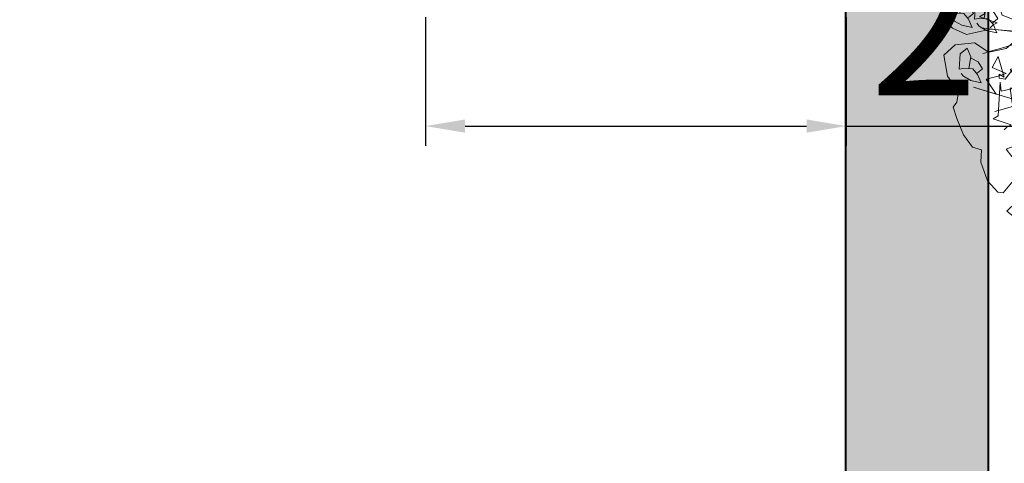
# Model space of a CAD drawing. Units: inches. Extents: x 2337 to 3570, y 1258 to 1938.
# Tile 8 of 30: x 2812 to 2874, y 1598 to 1626. Entities that reach past the tile are written whole.
import ezdxf

# ---------------------------------------------------------------- set-up
doc = ezdxf.new("R2010")
doc.units = ezdxf.units.IN
for name, color, linetype, lineweight in [('A-ANNO-DIMS', 2, 'Continuous', 18), ('A-WALL', 7, 'Continuous', 40), ('ARBOL', 74, 'Continuous', 13)]:
    doc.layers.add(name, color=color, linetype=linetype, lineweight=lineweight)
doc.layers.add('A-WALL-PATT', color=18, linetype='Continuous', lineweight=13, true_color=0x000000)
doc.layers.add('TALLO', color=36, linetype='Continuous')
doc.styles.get("Standard").update_dxf_attribs({"font": 'arial.ttf'})
doc.dimstyles.new('ISO-25', dxfattribs={"dimtxt": 9, "dimasz": 2.5, "dimexe": 1.25, "dimexo": 0.625, "dimtad": 1, "dimdec": 1, "dimlunit": 3, "dimtxsty": 'Standard', "dimcen": 2.5, "dimadec": 0, "dimazin": 0, "dimtfac": 1, "dimtdec": 1, "dimtmove": 0, "dimatfit": 3, "dimfxl": 1, "dimarcsym": 0})

# ---------------------------------------------------------------- blocks, each defined once
blk = doc.blocks.new('fresno')
at = {"layer": 'ARBOL'}
for p, q in [((2.96, 0.991), (3.575, 1.984)), ((-3.638, 1.194), (-4.164, 1.76)), ((-1.151, -0.932), (-1.99, -1.556)), ((-0.974, -3.757), (-1.31, -4.423))]:
    blk.add_line(p, q, dxfattribs=at)
blk.add_lwpolyline([(0.823, 4.745), (0.566, 4.764), (0.459, 4.687), (0.336, 4.518), (0.233, 4.322), (0.087, 4.298), (0.091, 4.464), (0.14, 4.621), (-0.09, 4.659), (-0.033, 4.863), (-0.264, 4.901), (-0.483, 4.866), (-0.686, 4.924), (-1.021, 4.801), (-1.288, 4.8), (-1.431, 4.563), (-1.234, 4.327), (-1.406, 4), (-1.205, 3.778), (-0.909, 3.705), (-0.931, 3.283), (-1.122, 2.983), (-1.491, 3.043), (-1.619, 3.562), (-1.9, 3.727), (-1.851, 3.982), (-2.197, 4.084), (-2.278, 4.31), (-2.543, 4.283), (-2.896, 4.152), (-3.091, 3.971), (-3.022, 3.817), (-3.244, 3.617), (-3.424, 3.528), (-3.697, 3.455), (-3.946, 3.236), (-3.922, 3.09), (-3.94, 2.548), (-3.617, 2.495), (-3.927, 2.19), (-4.062, 2.379), (-4.443, 2.512), (-4.546, 2.316), (-4.73, 2.062), (-4.767, 1.832), (-4.671, 1.698), (-4.486, 1.667), (-4.693, 1.559), (-4.854, 1.444), (-4.934, 1.102), (-5.037, 0.905), (-5.175, 0.644), (-5.166, 0.406), (-5.024, 0.264), (-4.781, 0.153), (-4.363, 0.249), (-4.014, 0.215), (-3.783, 0.177), (-3.46, 0.124), (-3.733, 0.051), (-4.132, -0.073), (-4.404, -0.146), (-4.639, 0.011), (-4.977, -0.028), (-5.172, -0.209), (-5.113, -0.574), (-4.921, -0.843), (-4.951, -1.027), (-5.012, -1.112), (-4.95, -1.311), (-4.83, -1.592), (-4.676, -1.807), (-4.518, -1.856), (-4.529, -2.068), (-4.417, -2.394), (-4.236, -2.59), (-4.143, -2.605), (-3.967, -2.397), (-3.703, -2.37), (-3.339, -2.027), (-3.032, -1.889), (-3.169, -2.15), (-3.115, -2.396), (-3.376, -2.542), (-3.552, -2.466), (-3.909, -2.762), (-4.077, -2.924), (-3.804, -3.135), (-3.592, -3.43), (-3.461, -3.499), (-3.253, -3.676), (-2.953, -3.867), (-2.792, -3.752), (-2.642, -3.848), (-2.572, -4.001), (-2.323, -4.066), (-2.18, -4.208), (-1.926, -4.392), (-1.58, -4.591), (-1.288, -4.545), (-1.027, -4.683), (-0.788, -4.675), (-0.531, -4.693), (-0.382, -4.505), (-0.29, -4.236), (-0.66, -3.891), (-0.588, -3.595), (-0.374, -3.441), (-0.267, -3.079), (-0.368, -2.541), (-0.208, -2.426), (-0.099, -2.633), (-0.087, -2.991), (0.071, -3.04), (0.129, -3.405), (-0.185, -3.59), (-0.119, -3.909), (0.055, -4.151), (0.136, -4.377), (0.456, -4.596), (0.828, -4.491), (1.227, -4.368), (1.461, -4.241), (1.583, -4.071), (1.748, -4.075), (1.86, -4.117), (2.101, -3.944), (2.308, -3.836), (2.925, -3.393), (3.101, -3.185), (2.74, -3.078), (2.812, -2.782), (2.769, -2.61), (3.015, -2.555), (3.012, -2.721), (3.254, -2.832), (3.546, -2.785), (3.752, -2.393), (3.882, -2.177), (3.92, -1.947), (4.069, -1.758), (4.214, -1.451), (4.144, -1.297), (4.021, -1.182), (4.182, -1.067), (4.304, -0.897), (4.464, -0.497), (4.429, -0.279), (4.406, -0.133), (3.964, -0.083), (3.074, -0.315), (2.582, -0.424), (2.217, -0.197), (2.136, 0.029), (2.462, 0.141), (2.628, -0.147), (3.012, -0.116), (3.249, 0.177), (3.602, 0.308), (3.701, 0.623), (4.089, 0.535), (4.404, 0.436), (4.464, 0.805), (4.272, 1.074), (4.267, 1.193), (4.336, 1.324), (4.243, 1.623), (4.092, 2.003), (3.769, 2.057), (3.485, 2.056), (3.642, 2.291), (3.88, 2.299), (3.71, 2.706), (3.563, 2.967), (3.201, 3.358), (3.001, 3.581), (2.766, 3.738), (2.635, 3.807), (2.332, 3.549), (2.268, 3.299), (2.052, 3.429), (2.136, 3.652), (1.798, 3.613), (1.437, 3.72), (1.755, 4.071), (1.513, 4.182), (1.451, 4.381), (1.519, 4.512), (1.204, 4.611), (1.012, 4.596)], close=True, dxfattribs=at)
for points in [[(-1.104, 4.45), (-1.063, 4.399), (-0.939, 4.325), (-0.757, 4.285), (-0.82, 4.431), (-0.903, 4.527), (-1.075, 4.533), (-1.143, 4.521), (-1.126, 4.792), (-1.002, 4.891), (-0.939, 4.738), (-0.975, 4.535)], [(-0.346, 4.735), (-0.501, 4.528), (-0.605, 4.545), (-0.605, 4.614), (-0.519, 4.563), (-0.622, 4.925), (-0.726, 4.735), (-0.484, 4.632), (-0.622, 4.58), (-0.829, 4.528), (-0.657, 4.27), (-1.053, 4.39), (-0.363, 4.183), (-0.381, 4.114), (-0.415, 4.373), (-0.26, 4.39), (-0.57, 4.321), (-0.588, 4.476), (-0.622, 3.89), (-0.708, 3.839), (-0.398, 3.735), (-0.467, 3.701), (-0.519, 3.649)], [(-0.935, 4.717), (-0.809, 4.65), (-0.736, 4.529), (-0.824, 4.459)], [(0.734, 4.203), (0.775, 4.152), (0.9, 4.078), (1.082, 4.038), (1.018, 4.185), (0.936, 4.281), (0.763, 4.287), (0.696, 4.274), (0.712, 4.546), (0.837, 4.645), (0.899, 4.491), (0.863, 4.289)], [(-0.521, 4.069), (-0.48, 4.018), (-0.356, 3.944), (-0.174, 3.904), (-0.237, 4.051), (-0.32, 4.146), (-0.492, 4.152), (-0.56, 4.14), (-0.543, 4.411), (-0.419, 4.511), (-0.356, 4.357), (-0.392, 4.154)], [(0.263, 4.114), (0.304, 4.063), (0.429, 3.989), (0.611, 3.948), (0.547, 4.095), (0.465, 4.191), (0.293, 4.197), (0.225, 4.185), (0.242, 4.456), (0.366, 4.555), (0.428, 4.402), (0.393, 4.199)], [(0.904, 4.471), (1.029, 4.404), (1.102, 4.282), (1.015, 4.212)], [(-1.623, 4.132), (-1.778, 3.925), (-1.882, 3.942), (-1.882, 4.011), (-1.795, 3.959), (-1.899, 4.321), (-2.002, 4.132), (-1.761, 4.028), (-1.899, 3.977), (-2.106, 3.925), (-1.933, 3.666), (-2.33, 3.787), (-1.64, 3.58), (-1.657, 3.511), (-1.692, 3.77), (-1.537, 3.787), (-1.847, 3.718), (-1.864, 3.873), (-1.899, 3.287), (-1.985, 3.235), (-1.675, 3.132), (-1.744, 3.097), (-1.795, 3.046)], [(-0.352, 4.337), (-0.226, 4.269), (-0.153, 4.148), (-0.241, 4.078)], [(0.433, 4.381), (0.558, 4.314), (0.631, 4.193), (0.544, 4.122)], [(-2.368, 4.073), (-2.523, 3.866), (-2.627, 3.883), (-2.627, 3.952), (-2.541, 3.9), (-2.644, 4.262), (-2.748, 4.073), (-2.506, 3.969), (-2.644, 3.918), (-2.851, 3.866), (-2.679, 3.607), (-3.075, 3.728), (-2.385, 3.521), (-2.403, 3.452), (-2.437, 3.711), (-2.282, 3.728), (-2.592, 3.659), (-2.61, 3.814), (-2.644, 3.228), (-2.73, 3.176), (-2.42, 3.073), (-2.489, 3.038), (-2.541, 2.987)], [(-2.629, 3.733), (-2.588, 3.682), (-2.463, 3.608), (-2.281, 3.568), (-2.345, 3.715), (-2.427, 3.81), (-2.6, 3.816), (-2.667, 3.804), (-2.651, 4.075), (-2.526, 4.175), (-2.464, 4.021), (-2.5, 3.818)], [(-1.149, 3.822), (-1.108, 3.771), (-0.983, 3.697), (-0.802, 3.657), (-0.865, 3.804), (-0.948, 3.9), (-1.12, 3.906), (-1.188, 3.893), (-1.171, 4.165), (-1.047, 4.264), (-0.984, 4.111), (-1.02, 3.908)], [(0.413, 4.08), (0.258, 3.873), (0.154, 3.89), (0.154, 3.959), (0.241, 3.908), (0.137, 4.27), (0.034, 4.08), (0.275, 3.977), (0.137, 3.925), (-0.07, 3.873), (0.103, 3.614), (-0.294, 3.735), (0.396, 3.528), (0.379, 3.459), (0.344, 3.718), (0.499, 3.735), (0.189, 3.666), (0.172, 3.821), (0.137, 3.235), (0.051, 3.183), (0.361, 3.08), (0.292, 3.046), (0.241, 2.994)], [(1.189, 3.942), (1.034, 3.735), (0.931, 3.752), (0.931, 3.821), (1.017, 3.77), (0.913, 4.132), (0.81, 3.942), (1.051, 3.839), (0.913, 3.787), (0.706, 3.735), (0.879, 3.477), (0.482, 3.597), (1.172, 3.39), (1.155, 3.321), (1.12, 3.58), (1.276, 3.597), (0.965, 3.528), (0.948, 3.683), (0.913, 3.097), (0.827, 3.046), (1.138, 2.942), (1.069, 2.908), (1.017, 2.856)], [(1.259, 4.08), (1.103, 3.873), (1, 3.89), (1, 3.959), (1.086, 3.908), (0.982, 4.27), (0.879, 4.08), (1.12, 3.977), (0.982, 3.925), (0.775, 3.873), (0.948, 3.614), (0.551, 3.735), (1.241, 3.528), (1.224, 3.459), (1.189, 3.718), (1.345, 3.735), (1.034, 3.666), (1.017, 3.821), (0.982, 3.235), (0.896, 3.183), (1.207, 3.08), (1.138, 3.046), (1.086, 2.994)], [(-2.459, 4), (-2.334, 3.933), (-2.261, 3.812), (-2.348, 3.742)], [(-0.287, 3.833), (-0.442, 3.626), (-0.546, 3.643), (-0.546, 3.712), (-0.46, 3.661), (-0.563, 4.023), (-0.667, 3.833), (-0.425, 3.73), (-0.563, 3.678), (-0.77, 3.626), (-0.598, 3.367), (-0.995, 3.488), (-0.304, 3.281), (-0.322, 3.212), (-0.356, 3.471), (-0.201, 3.488), (-0.511, 3.419), (-0.529, 3.574), (-0.563, 2.988), (-0.649, 2.936), (-0.339, 2.833), (-0.408, 2.799), (-0.46, 2.747)], [(-0.98, 4.09), (-0.854, 4.023), (-0.781, 3.901), (-0.869, 3.831)], [(1.25, 3.643), (1.291, 3.592), (1.416, 3.518), (1.597, 3.478), (1.534, 3.625), (1.451, 3.721), (1.279, 3.727), (1.211, 3.714), (1.228, 3.985), (1.352, 4.085), (1.415, 3.931), (1.379, 3.729)], [(-1.951, 3.597), (-2.106, 3.39), (-2.209, 3.408), (-2.209, 3.477), (-2.123, 3.425), (-2.227, 3.787), (-2.33, 3.597), (-2.089, 3.494), (-2.227, 3.442), (-2.434, 3.39), (-2.261, 3.132), (-2.658, 3.252), (-1.968, 3.046), (-1.985, 2.977), (-2.02, 3.235), (-1.864, 3.252), (-2.175, 3.183), (-2.192, 3.339), (-2.227, 2.752), (-2.313, 2.701), (-2.002, 2.597), (-2.071, 2.563), (-2.123, 2.511)], [(-2.068, 3.464), (-2.027, 3.413), (-1.903, 3.339), (-1.721, 3.299), (-1.784, 3.446), (-1.867, 3.542), (-2.039, 3.547), (-2.107, 3.535), (-2.09, 3.806), (-1.966, 3.906), (-1.903, 3.752), (-1.939, 3.55)], [(0.837, 2.414), (0.533, 3.352), (0.697, 3.906)], [(1.419, 3.911), (1.545, 3.844), (1.618, 3.722), (1.53, 3.652)], [(-2.898, 3.511), (-3.053, 3.304), (-3.157, 3.321), (-3.157, 3.39), (-3.071, 3.339), (-3.174, 3.701), (-3.278, 3.511), (-3.036, 3.408), (-3.174, 3.356), (-3.381, 3.304), (-3.209, 3.046), (-3.605, 3.166), (-2.915, 2.959), (-2.932, 2.89), (-2.967, 3.149), (-2.812, 3.166), (-3.122, 3.097), (-3.14, 3.253), (-3.174, 2.666), (-3.26, 2.615), (-2.95, 2.511), (-3.019, 2.477), (-3.071, 2.425)], [(-1.899, 3.732), (-1.773, 3.664), (-1.7, 3.543), (-1.788, 3.473)], [(-0.063, 3.671), (-0.069, 3.151), (-0.364, 2.965), (-0.319, 2.449)], [(1.259, 2.882), (1.254, 3.446), (1.381, 3.636)], [(-3.413, 3.083), (-3.373, 3.032), (-3.248, 2.958), (-3.066, 2.918), (-3.129, 3.065), (-3.212, 3.161), (-3.384, 3.167), (-3.452, 3.154), (-3.435, 3.425), (-3.311, 3.525), (-3.248, 3.371), (-3.284, 3.169)], [(-1.367, 2.367), (-1.081, 2.78), (-1.193, 3.514)], [(-0.923, 3.449), (-0.951, 3.425), (-0.93, 3.313)], [(-0.358, 2.895), (-0.615, 3.037), (-0.783, 3.596)], [(0.558, 3.402), (0.403, 3.195), (0.299, 3.212), (0.299, 3.281), (0.386, 3.23), (0.282, 3.592), (0.179, 3.402), (0.42, 3.299), (0.282, 3.247), (0.075, 3.195), (0.248, 2.936), (-0.149, 3.057), (0.541, 2.85), (0.524, 2.781), (0.489, 3.04), (0.644, 3.057), (0.334, 2.988), (0.317, 3.143), (0.282, 2.557), (0.196, 2.505), (0.506, 2.402), (0.437, 2.368), (0.386, 2.316)], [(1.564, 3.016), (1.605, 2.965), (1.729, 2.891), (1.911, 2.851), (1.848, 2.998), (1.765, 3.094), (1.593, 3.099), (1.525, 3.087), (1.542, 3.358), (1.666, 3.458), (1.729, 3.304), (1.693, 3.102)], [(2.191, 3.038), (2.232, 2.987), (2.357, 2.913), (2.539, 2.873), (2.475, 3.02), (2.393, 3.116), (2.221, 3.122), (2.153, 3.109), (2.17, 3.381), (2.294, 3.48), (2.356, 3.326), (2.321, 3.124)], [(2.573, 3.128), (2.613, 3.077), (2.738, 3.003), (2.92, 2.963), (2.857, 3.11), (2.774, 3.205), (2.602, 3.211), (2.534, 3.199), (2.551, 3.47), (2.675, 3.57), (2.738, 3.416), (2.702, 3.214)], [(-3.244, 3.351), (-3.118, 3.284), (-3.045, 3.162), (-3.133, 3.092)], [(-0.448, 1), (-0.961, 1.419), (-1.784, 3.341)], [(-0.41, 3.035), (-0.387, 2.974), (-0.291, 2.865), (-0.131, 2.771), (-0.146, 2.93), (-0.195, 3.047), (-0.357, 3.106), (-0.425, 3.115), (-0.325, 3.368), (-0.176, 3.424), (-0.164, 3.258), (-0.261, 3.077)], [(0.746, 2.242), (1.034, 2.786), (1.584, 3.019), (1.879, 3.374)], [(1.733, 3.284), (1.859, 3.216), (1.932, 3.095), (1.844, 3.025)], [(2.361, 3.306), (2.486, 3.239), (2.559, 3.117), (2.472, 3.047)], [(2.742, 3.396), (2.868, 3.328), (2.941, 3.207), (2.853, 3.137)], [(3.111, 2.904), (3.152, 2.853), (3.276, 2.779), (3.458, 2.739), (3.395, 2.886), (3.312, 2.981), (3.14, 2.987), (3.072, 2.975), (3.089, 3.246), (3.213, 3.346), (3.276, 3.192), (3.24, 2.99)], [(-2.225, 2.77), (-2.184, 2.718), (-2.06, 2.645), (-1.878, 2.604), (-1.941, 2.751), (-2.024, 2.847), (-2.196, 2.853), (-2.264, 2.84), (-2.247, 3.112), (-2.123, 3.211), (-2.06, 3.058), (-2.096, 2.855)], [(-1.575, 2.854), (-2.052, 2.969), (-2.2, 3.178)], [(-1.373, 2.77), (-1.332, 2.718), (-1.208, 2.645), (-1.026, 2.604), (-1.089, 2.751), (-1.172, 2.847), (-1.344, 2.853), (-1.412, 2.84), (-1.395, 3.112), (-1.271, 3.211), (-1.208, 3.058), (-1.244, 2.855)], [(-0.166, 3.238), (-0.068, 3.135), (-0.036, 2.997), (-0.141, 2.957)], [(2.326, 2.702), (2.367, 2.651), (2.492, 2.577), (2.673, 2.537), (2.61, 2.684), (2.527, 2.78), (2.355, 2.786), (2.287, 2.773), (2.304, 3.045), (2.428, 3.144), (2.491, 2.99), (2.455, 2.788)], [(3.28, 3.172), (3.406, 3.104), (3.479, 2.983), (3.391, 2.913)], [(-3.434, 2.752), (-3.59, 2.546), (-3.693, 2.563), (-3.693, 2.632), (-3.607, 2.58), (-3.71, 2.942), (-3.814, 2.752), (-3.572, 2.649), (-3.71, 2.597), (-3.917, 2.546), (-3.745, 2.287), (-4.142, 2.408), (-3.452, 2.201), (-3.469, 2.132), (-3.503, 2.39), (-3.348, 2.408), (-3.659, 2.339), (-3.676, 2.494), (-3.71, 1.908), (-3.797, 1.856), (-3.486, 1.753), (-3.555, 1.718), (-3.607, 1.666)], [(-1.112, 1.773), (-2.014, 2.265), (-2.654, 2.957)], [(-2.056, 3.037), (-1.93, 2.97), (-1.857, 2.849), (-1.945, 2.778)], [(-0.57, 2.77), (-0.726, 2.563), (-0.829, 2.58), (-0.829, 2.649), (-0.743, 2.597), (-0.846, 2.959), (-0.95, 2.77), (-0.708, 2.666), (-0.846, 2.615), (-1.053, 2.563), (-0.881, 2.304), (-1.278, 2.425), (-0.588, 2.218), (-0.605, 2.149), (-0.639, 2.408), (-0.484, 2.425), (-0.795, 2.356), (-0.812, 2.511), (-0.846, 1.925), (-0.933, 1.873), (-0.622, 1.77), (-0.691, 1.735), (-0.743, 1.684)], [(-1.204, 3.037), (-1.078, 2.97), (-1.005, 2.849), (-1.093, 2.778)], [(2.121, 2.804), (1.966, 2.597), (1.862, 2.615), (1.862, 2.683), (1.949, 2.632), (1.845, 2.994), (1.742, 2.804), (1.983, 2.701), (1.845, 2.649), (1.638, 2.597), (1.811, 2.339), (1.414, 2.459), (2.104, 2.252), (2.087, 2.184), (2.052, 2.442), (2.207, 2.459), (1.897, 2.39), (1.88, 2.546), (1.845, 1.959), (1.759, 1.908), (2.069, 1.804), (2, 1.77), (1.949, 1.718)], [(2.495, 2.97), (2.621, 2.903), (2.694, 2.781), (2.606, 2.711)], [(3.043, 2.478), (3.084, 2.427), (3.209, 2.353), (3.391, 2.313), (3.327, 2.46), (3.245, 2.556), (3.073, 2.562), (3.005, 2.549), (3.022, 2.82), (3.146, 2.92), (3.208, 2.766), (3.173, 2.564)], [(2.171, 1.674), (2.121, 2.172), (2.689, 2.898)], [(3.519, 2.666), (3.363, 2.459), (3.26, 2.477), (3.26, 2.546), (3.346, 2.494), (3.243, 2.856), (3.139, 2.666), (3.381, 2.563), (3.243, 2.511), (3.036, 2.459), (3.208, 2.201), (2.811, 2.321), (3.501, 2.115), (3.484, 2.046), (3.45, 2.304), (3.605, 2.321), (3.294, 2.252), (3.277, 2.408), (3.243, 1.821), (3.156, 1.77), (3.467, 1.666), (3.398, 1.632), (3.346, 1.58)], [(3.213, 2.746), (3.338, 2.679), (3.411, 2.557), (3.324, 2.487)], [(1.586, 2.528), (1.431, 2.321), (1.327, 2.339), (1.327, 2.408), (1.414, 2.356), (1.31, 2.718), (1.207, 2.528), (1.448, 2.425), (1.31, 2.373), (1.103, 2.321), (1.276, 2.063), (0.879, 2.184), (1.569, 1.977), (1.552, 1.908), (1.517, 2.166), (1.673, 2.184), (1.362, 2.115), (1.345, 2.27), (1.31, 1.684), (1.224, 1.632), (1.535, 1.528), (1.466, 1.494), (1.414, 1.442)], [(3.178, 2.165), (3.219, 2.113), (3.344, 2.04), (3.525, 1.999), (3.462, 2.146), (3.379, 2.242), (3.207, 2.248), (3.139, 2.236), (3.156, 2.507), (3.28, 2.606), (3.343, 2.453), (3.307, 2.25)], [(-4.422, 2.03), (-4.381, 1.979), (-4.257, 1.905), (-4.075, 1.865), (-4.138, 2.012), (-4.221, 2.108), (-4.393, 2.114), (-4.461, 2.101), (-4.444, 2.372), (-4.32, 2.472), (-4.257, 2.318), (-4.293, 2.116)], [(-3.468, 1.85), (-3.409, 2.222), (-3.628, 2.505)], [(-1.817, 2.351), (-1.972, 2.144), (-2.075, 2.162), (-2.075, 2.231), (-1.989, 2.179), (-2.093, 2.541), (-2.196, 2.351), (-1.955, 2.248), (-2.093, 2.196), (-2.3, 2.144), (-2.127, 1.886), (-2.524, 2.006), (-1.834, 1.8), (-1.851, 1.731), (-1.886, 1.989), (-1.73, 2.006), (-2.041, 1.937), (-2.058, 2.093), (-2.093, 1.506), (-2.179, 1.455), (-1.868, 1.351), (-1.937, 1.317), (-1.989, 1.265)], [(-1.786, 2.007), (-1.722, 1.99), (-1.578, 2.003), (-1.407, 2.078), (-1.545, 2.159), (-1.668, 2.188), (-1.811, 2.092), (-1.859, 2.042), (-2.004, 2.271), (-1.962, 2.425), (-1.821, 2.337), (-1.731, 2.152)], [(3.245, 1.963), (3.286, 1.912), (3.411, 1.838), (3.593, 1.798), (3.529, 1.945), (3.447, 2.041), (3.274, 2.046), (3.206, 2.034), (3.223, 2.305), (3.347, 2.405), (3.41, 2.251), (3.374, 2.049)], [(3.347, 2.432), (3.473, 2.365), (3.546, 2.244), (3.458, 2.173)], [(-3.986, 2.149), (-4.142, 1.942), (-4.245, 1.959), (-4.245, 2.028), (-4.159, 1.977), (-4.262, 2.339), (-4.366, 2.149), (-4.124, 2.046), (-4.262, 1.994), (-4.47, 1.942), (-4.297, 1.684), (-4.694, 1.804), (-4.004, 1.597), (-4.021, 1.528), (-4.055, 1.787), (-3.9, 1.804), (-4.211, 1.735), (-4.228, 1.89), (-4.262, 1.304), (-4.349, 1.253), (-4.038, 1.149), (-4.107, 1.115), (-4.159, 1.063)], [(-4.253, 2.298), (-4.127, 2.231), (-4.054, 2.109), (-4.142, 2.039)], [(-3.533, 2.149), (-3.43, 2.247), (-3.292, 2.279), (-3.252, 2.174)], [(-1.806, 2.323), (-1.665, 2.343), (-1.534, 2.287), (-1.564, 2.179)], [(-0.566, 1.873), (-0.525, 1.822), (-0.4, 1.748), (-0.219, 1.708), (-0.282, 1.855), (-0.365, 1.951), (-0.537, 1.957), (-0.605, 1.944), (-0.588, 2.216), (-0.464, 2.315), (-0.401, 2.162), (-0.437, 1.959)], [(3.415, 2.231), (3.54, 2.163), (3.613, 2.042), (3.525, 1.972)], [(-2.916, 0.958), (-3.096, 1.528), (-3.871, 2.197)], [(-3.331, 1.905), (-3.269, 1.928), (-3.161, 2.024), (-3.066, 2.184), (-3.226, 2.169), (-3.342, 2.121), (-3.401, 1.958), (-3.41, 1.89), (-3.663, 1.99), (-3.719, 2.139), (-3.554, 2.151), (-3.372, 2.054)], [(-1.164, 1.612), (-1.109, 1.576), (-0.967, 1.544), (-0.782, 1.562), (-0.888, 1.682), (-0.996, 1.748), (-1.162, 1.7), (-1.222, 1.667), (-1.29, 1.93), (-1.203, 2.063), (-1.096, 1.937), (-1.067, 1.733)], [(-0.397, 2.141), (-0.271, 2.074), (-0.198, 1.952), (-0.286, 1.882)], [(0.72, 1.798), (0.723, 1.733), (0.781, 1.6), (0.904, 1.46), (0.939, 1.616), (0.929, 1.742), (0.793, 1.848), (0.73, 1.878), (0.904, 2.088), (1.062, 2.095), (1.023, 1.934), (0.875, 1.791)], [(-2.965, 1.493), (-2.924, 1.441), (-2.799, 1.368), (-2.618, 1.327), (-2.681, 1.474), (-2.764, 1.57), (-2.936, 1.576), (-3.004, 1.564), (-2.987, 1.835), (-2.863, 1.934), (-2.8, 1.781), (-2.836, 1.578)], [(-1.085, 1.919), (-0.945, 1.893), (-0.838, 1.801), (-0.9, 1.707)], [(1.014, 1.915), (1.077, 1.787), (1.064, 1.646), (0.952, 1.64)], [(3.649, 1.515), (3.69, 1.464), (3.814, 1.39), (3.996, 1.35), (3.933, 1.497), (3.85, 1.592), (3.678, 1.598), (3.61, 1.586), (3.627, 1.857), (3.751, 1.957), (3.814, 1.803), (3.778, 1.601)], [(3.716, 1.537), (3.757, 1.486), (3.882, 1.412), (4.063, 1.372), (4, 1.519), (3.917, 1.615), (3.745, 1.621), (3.677, 1.608), (3.694, 1.88), (3.818, 1.979), (3.881, 1.825), (3.845, 1.623)], [(-2.796, 1.76), (-2.67, 1.693), (-2.597, 1.572), (-2.685, 1.501)], [(2.587, 1.684), (2.432, 1.477), (2.328, 1.494), (2.328, 1.563), (2.414, 1.511), (2.311, 1.873), (2.207, 1.684), (2.449, 1.58), (2.311, 1.528), (2.104, 1.477), (2.276, 1.218), (1.88, 1.339), (2.57, 1.132), (2.552, 1.063), (2.518, 1.321), (2.673, 1.339), (2.363, 1.27), (2.345, 1.425), (2.311, 0.839), (2.225, 0.787), (2.535, 0.684), (2.466, 0.649), (2.414, 0.597)], [(3.818, 1.783), (3.944, 1.715), (4.017, 1.594), (3.929, 1.524)], [(3.885, 1.805), (4.011, 1.738), (4.084, 1.616), (3.996, 1.546)], [(-4.193, 1.356), (-4.349, 1.149), (-4.452, 1.166), (-4.452, 1.235), (-4.366, 1.184), (-4.469, 1.546), (-4.573, 1.356), (-4.331, 1.253), (-4.469, 1.201), (-4.677, 1.149), (-4.504, 0.89), (-4.901, 1.011), (-4.211, 0.804), (-4.228, 0.735), (-4.262, 0.994), (-4.107, 1.011), (-4.418, 0.942), (-4.435, 1.097), (-4.469, 0.511), (-4.556, 0.459), (-4.245, 0.356), (-4.314, 0.322), (-4.366, 0.27)], [(-4.759, 1.269), (-4.718, 1.217), (-4.593, 1.144), (-4.411, 1.103), (-4.475, 1.25), (-4.557, 1.346), (-4.729, 1.352), (-4.797, 1.339), (-4.78, 1.611), (-4.656, 1.71), (-4.594, 1.557), (-4.629, 1.354)], [(-1.575, 1.269), (-1.534, 1.217), (-1.409, 1.144), (-1.228, 1.103), (-1.291, 1.25), (-1.373, 1.346), (-1.546, 1.352), (-1.614, 1.339), (-1.597, 1.611), (-1.473, 1.71), (-1.41, 1.557), (-1.446, 1.354)], [(1.283, 1.469), (1.266, 1.405), (1.279, 1.261), (1.354, 1.09), (1.435, 1.228), (1.464, 1.351), (1.368, 1.494), (1.318, 1.542), (1.547, 1.687), (1.7, 1.645), (1.613, 1.504), (1.428, 1.414)], [(3.761, 1.112), (3.802, 1.061), (3.926, 0.987), (4.108, 0.947), (4.045, 1.093), (3.962, 1.189), (3.79, 1.195), (3.722, 1.183), (3.739, 1.454), (3.863, 1.553), (3.926, 1.4), (3.89, 1.197)], [(-4.589, 1.536), (-4.464, 1.469), (-4.391, 1.348), (-4.478, 1.277)], [(-1.406, 1.536), (-1.28, 1.469), (-1.207, 1.348), (-1.295, 1.277)], [(0.308, 0.933), (0.349, 0.881), (0.474, 0.807), (0.656, 0.767), (0.592, 0.914), (0.51, 1.01), (0.337, 1.016), (0.27, 1.003), (0.286, 1.275), (0.411, 1.374), (0.473, 1.221), (0.437, 1.018)], [(1.599, 1.489), (1.618, 1.348), (1.563, 1.217), (1.455, 1.247)], [(2.479, 1.34), (2.443, 1.285), (2.411, 1.143), (2.429, 0.958), (2.549, 1.064), (2.615, 1.172), (2.567, 1.338), (2.534, 1.398), (2.797, 1.466), (2.93, 1.379), (2.804, 1.272), (2.6, 1.243)], [(3.139, 1.235), (2.984, 1.028), (2.88, 1.046), (2.88, 1.115), (2.967, 1.063), (2.863, 1.425), (2.759, 1.235), (3.001, 1.132), (2.863, 1.08), (2.656, 1.028), (2.828, 0.77), (2.432, 0.891), (3.122, 0.684), (3.105, 0.615), (3.07, 0.873), (3.225, 0.891), (2.915, 0.822), (2.897, 0.977), (2.863, 0.391), (2.777, 0.339), (3.087, 0.235), (3.018, 0.201), (2.967, 0.149)], [(3.93, 1.379), (4.056, 1.312), (4.129, 1.191), (4.041, 1.121)], [(-3.192, 1.017), (-3.578, 1.215), (-3.949, 1.081), (-4.398, 1.339)], [(-3.481, 0.843), (-3.44, 0.792), (-3.315, 0.718), (-3.133, 0.678), (-3.197, 0.825), (-3.279, 0.92), (-3.451, 0.926), (-3.519, 0.914), (-3.502, 1.185), (-3.378, 1.285), (-3.316, 1.131), (-3.351, 0.928)], [(-2.703, 1.201), (-2.575, 1.263), (-2.433, 1.251), (-2.428, 1.139)], [(2.786, 1.261), (2.76, 1.121), (2.668, 1.014), (2.574, 1.076)], [(4.01, 1.36), (3.422, 0.918)], [(4.26, 1.115), (4.105, 0.908), (4.002, 0.925), (4.002, 0.994), (4.088, 0.942), (3.984, 1.304), (3.881, 1.115), (4.122, 1.011), (3.984, 0.959), (3.777, 0.908), (3.95, 0.649), (3.553, 0.77), (4.243, 0.563), (4.226, 0.494), (4.191, 0.753), (4.347, 0.77), (4.036, 0.701), (4.019, 0.856), (3.984, 0.27), (3.898, 0.218), (4.209, 0.115), (4.14, 0.08), (4.088, 0.029)], [(-3.354, 1.176), (-4.529, 0.864)], [(-3.311, 1.111), (-3.186, 1.043), (-3.113, 0.922), (-3.2, 0.852)], [(0.478, 1.2), (0.603, 1.133), (0.676, 1.011), (0.589, 0.941)], [(2.808, 1.015), (3.422, 0.918), (3.422, 0.918), (3.748, 0.794), (4.154, 1.111)], [(-5.028, 0.44), (-4.987, 0.388), (-4.862, 0.315), (-4.68, 0.274), (-4.744, 0.421), (-4.826, 0.517), (-4.998, 0.523), (-5.066, 0.511), (-5.049, 0.782), (-4.925, 0.881), (-4.863, 0.728), (-4.898, 0.525)], [(-1.981, 0.615), (-1.915, 0.618), (-1.782, 0.676), (-1.643, 0.799), (-1.799, 0.834), (-1.925, 0.824), (-2.031, 0.688), (-2.061, 0.626), (-2.27, 0.799), (-2.278, 0.958), (-2.117, 0.918), (-1.974, 0.77)], [(-0.397, 0.517), (-0.346, 0.557), (-0.272, 0.682), (-0.232, 0.864), (-0.379, 0.801), (-0.474, 0.718), (-0.48, 0.546), (-0.468, 0.478), (-0.739, 0.495), (-0.838, 0.619), (-0.685, 0.682), (-0.482, 0.646)], [(4.075, 0.529), (4.116, 0.478), (4.24, 0.404), (4.422, 0.364), (4.359, 0.511), (4.276, 0.607), (4.104, 0.613), (4.036, 0.6), (4.053, 0.871), (4.177, 0.971), (4.24, 0.817), (4.204, 0.615)], [(-4.858, 0.707), (-4.733, 0.64), (-4.66, 0.519), (-4.747, 0.448)], [(-4.602, 0.35), (-4.561, 0.299), (-4.436, 0.225), (-4.254, 0.185), (-4.318, 0.332), (-4.4, 0.428), (-4.572, 0.433), (-4.64, 0.421), (-4.623, 0.692), (-4.499, 0.792), (-4.437, 0.638), (-4.472, 0.436)], [(-2.698, 0.509), (-2.854, 0.302), (-2.957, 0.319), (-2.957, 0.388), (-2.871, 0.336), (-2.974, 0.698), (-3.078, 0.509), (-2.836, 0.405), (-2.974, 0.353), (-3.182, 0.302), (-3.009, 0.043), (-3.406, 0.164), (-2.716, -0.043), (-2.733, -0.112), (-2.767, 0.147), (-2.612, 0.164), (-2.923, 0.095), (-2.94, 0.25), (-2.974, -0.336), (-3.061, -0.388), (-2.75, -0.491), (-2.819, -0.526), (-2.871, -0.577)], [(2.639, 0.58), (2.483, 0.373), (2.38, 0.391), (2.38, 0.46), (2.466, 0.408), (2.363, 0.77), (2.259, 0.58), (2.501, 0.477), (2.363, 0.425), (2.156, 0.373), (2.328, 0.115), (1.931, 0.235), (2.621, 0.029), (2.604, -0.04), (2.57, 0.218), (2.725, 0.235), (2.414, 0.166), (2.397, 0.322), (2.363, -0.265), (2.276, -0.316), (2.587, -0.42), (2.518, -0.454), (2.466, -0.506)], [(2.708, 0.563), (2.552, 0.356), (2.449, 0.373), (2.449, 0.442), (2.535, 0.391), (2.432, 0.753), (2.328, 0.563), (2.57, 0.46), (2.432, 0.408), (2.225, 0.356), (2.397, 0.097), (2, 0.218), (2.69, 0.011), (2.673, -0.058), (2.639, 0.201), (2.794, 0.218), (2.483, 0.149), (2.466, 0.304), (2.432, -0.282), (2.345, -0.334), (2.656, -0.437), (2.587, -0.471), (2.535, -0.523)], [(4.244, 0.797), (4.37, 0.73), (4.443, 0.608), (4.355, 0.538)], [(-4.432, 0.618), (-4.307, 0.55), (-4.234, 0.429), (-4.321, 0.359)], [(-3.824, 0.404), (-3.763, 0.427), (-3.654, 0.523), (-3.559, 0.683), (-3.719, 0.668), (-3.835, 0.62), (-3.894, 0.457), (-3.903, 0.389), (-4.156, 0.489), (-4.212, 0.638), (-4.047, 0.65), (-3.865, 0.553)], [(-2.322, 0.222), (-2.219, 0.321), (-2.081, 0.353), (-2.042, 0.248)], [(1.978, 0.384), (1.927, 0.343), (1.853, 0.218), (1.813, 0.036), (1.96, 0.1), (2.056, 0.182), (2.061, 0.355), (2.049, 0.422), (2.32, 0.406), (2.42, 0.281), (2.266, 0.219), (2.064, 0.254)], [(3.829, 0.184), (3.674, -0.023), (3.57, -0.006), (3.57, 0.063), (3.657, 0.011), (3.553, 0.373), (3.45, 0.184), (3.691, 0.08), (3.553, 0.029), (3.346, -0.023), (3.519, -0.282), (3.122, -0.161), (3.812, -0.368), (3.795, -0.437), (3.76, -0.178), (3.915, -0.161), (3.605, -0.23), (3.588, -0.075), (3.553, -0.661), (3.467, -0.713), (3.777, -0.816), (3.708, -0.851), (3.657, -0.902)], [(-3.394, 0.18), (-3.77, 0.182), (-4.532, 0.27)], [(-3.77, 0.182), (-4.09, -0.088), (-4.494, -0.18)], [(-0.596, -0.564), (0.03, -0.026), (0.339, 0.235)], [(2.246, 0.214), (2.178, 0.089), (2.057, 0.016), (1.987, 0.103)], [(-1.642, -0.412), (-1.601, -0.463), (-1.477, -0.537), (-1.295, -0.577), (-1.358, -0.43), (-1.441, -0.334), (-1.613, -0.328), (-1.681, -0.341), (-1.664, -0.069), (-1.54, 0.03), (-1.477, -0.124), (-1.513, -0.326)], [(0.03, -0.026), (-0.491, 0.154), (-0.871, -0.08)], [(0.38, 0.131), (0.248, -0.21), (-0.33, -0.951)], [(-4.871, -0.524), (-4.83, -0.575), (-4.705, -0.649), (-4.523, -0.689), (-4.587, -0.542), (-4.669, -0.446), (-4.841, -0.44), (-4.909, -0.453), (-4.893, -0.181), (-4.768, -0.082), (-4.706, -0.236), (-4.741, -0.438)], [(-1.473, -0.144), (-1.347, -0.211), (-1.274, -0.333), (-1.362, -0.403)], [(3.139, -0.282), (2.984, -0.489), (2.88, -0.471), (2.88, -0.402), (2.967, -0.454), (2.863, -0.092), (2.759, -0.282), (3.001, -0.385), (2.863, -0.437), (2.656, -0.489), (2.828, -0.747), (2.432, -0.627), (3.122, -0.834), (3.105, -0.902), (3.07, -0.644), (3.225, -0.627), (2.915, -0.696), (2.897, -0.54), (2.863, -1.127), (2.777, -1.178), (3.087, -1.282), (3.018, -1.316), (2.967, -1.368)], [(-4.701, -0.256), (-4.576, -0.323), (-4.503, -0.445), (-4.59, -0.515)], [(-3.952, -0.42), (-4.107, -0.627), (-4.211, -0.609), (-4.211, -0.54), (-4.124, -0.592), (-4.228, -0.23), (-4.331, -0.42), (-4.09, -0.523), (-4.228, -0.575), (-4.435, -0.627), (-4.262, -0.885), (-4.659, -0.765), (-3.969, -0.971), (-3.986, -1.04), (-4.021, -0.782), (-3.866, -0.765), (-4.176, -0.834), (-4.193, -0.678), (-4.228, -1.265), (-4.314, -1.316), (-4.004, -1.42), (-4.073, -1.454), (-4.124, -1.506)], [(-3.58, -0.559), (-3.529, -0.518), (-3.455, -0.393), (-3.415, -0.211), (-3.562, -0.275), (-3.658, -0.357), (-3.664, -0.53), (-3.651, -0.597), (-3.923, -0.581), (-4.022, -0.456), (-3.868, -0.394), (-3.666, -0.43)], [(-3.848, -0.389), (-3.781, -0.264), (-3.659, -0.191), (-3.589, -0.278)], [(1.822, -0.495), (2.859, -1.165)], [(1.846, -0.51), (2.605, -0.469), (3.129, -0.637)], [(-3.141, -0.713), (-3.296, -0.92), (-3.4, -0.902), (-3.4, -0.834), (-3.314, -0.885), (-3.417, -0.523), (-3.521, -0.713), (-3.279, -0.816), (-3.417, -0.868), (-3.624, -0.92), (-3.452, -1.178), (-3.848, -1.058), (-3.158, -1.265), (-3.175, -1.333), (-3.21, -1.075), (-3.055, -1.058), (-3.365, -1.127), (-3.383, -0.971), (-3.417, -1.558), (-3.503, -1.609), (-3.193, -1.713), (-3.262, -1.747), (-3.314, -1.799)], [(1.304, -0.681), (1.241, -0.664), (1.097, -0.678), (0.926, -0.752), (1.064, -0.833), (1.187, -0.862), (1.33, -0.766), (1.377, -0.716), (1.523, -0.945), (1.481, -1.099), (1.34, -1.011), (1.25, -0.826)], [(-3.195, -0.824), (-3.267, -0.898), (-4.285, -1.185)], [(-1.047, -0.767), (-1.151, -0.913), (-1.144, -1.307), (-1.61, -1.871)], [(-1.794, -1.268), (-1.758, -1.214), (-1.726, -1.072), (-1.744, -0.887), (-1.865, -0.993), (-1.93, -1.101), (-1.883, -1.266), (-1.85, -1.327), (-2.113, -1.395), (-2.246, -1.307), (-2.119, -1.2), (-1.916, -1.172)], [(-2.101, -1.19), (-2.076, -1.05), (-1.983, -0.943), (-1.889, -1.004)], [(-0.346, -1.024), (-1.05, -2.251)], [(1.903, -0.903), (1.837, -0.905), (1.704, -0.963), (1.565, -1.086), (1.721, -1.122), (1.847, -1.111), (1.953, -0.975), (1.983, -0.913), (2.192, -1.086), (2.2, -1.245), (2.039, -1.205), (1.896, -1.057)], [(0.748, -1.185), (1.452, -1.855), (2.021, -2.292)], [(2.02, -1.197), (1.891, -1.259), (1.75, -1.247), (1.745, -1.134)], [(3.253, -1.094), (3.192, -1.117), (3.083, -1.213), (2.988, -1.374), (3.148, -1.359), (3.264, -1.31), (3.323, -1.148), (3.332, -1.079), (3.585, -1.179), (3.641, -1.328), (3.476, -1.34), (3.294, -1.244)], [(3.105, -1.471), (2.949, -1.678), (2.846, -1.661), (2.846, -1.592), (2.932, -1.644), (2.829, -1.282), (2.725, -1.471), (2.967, -1.575), (2.829, -1.627), (2.621, -1.678), (2.794, -1.937), (2.397, -1.816), (3.087, -2.023), (3.07, -2.092), (3.036, -1.833), (3.191, -1.816), (2.88, -1.885), (2.863, -1.73), (2.829, -2.316), (2.742, -2.368), (3.053, -2.471), (2.984, -2.506), (2.932, -2.558)], [(3.455, -1.338), (3.352, -1.437), (3.214, -1.469), (3.175, -1.364)], [(-1.361, -1.756), (-1.343, -1.693), (-1.357, -1.548), (-1.431, -1.377), (-1.513, -1.515), (-1.542, -1.638), (-1.445, -1.781), (-1.395, -1.829), (-1.625, -1.974), (-1.778, -1.932), (-1.691, -1.791), (-1.506, -1.701)], [(-1.677, -1.776), (-1.696, -1.635), (-1.641, -1.504), (-1.533, -1.534)], [(-3.648, -1.948), (-3.596, -1.907), (-3.523, -1.782), (-3.482, -1.6), (-3.629, -1.664), (-3.725, -1.746), (-3.731, -1.919), (-3.719, -1.986), (-3.99, -1.97), (-4.089, -1.845), (-3.936, -1.783), (-3.733, -1.819)], [(-3.915, -1.778), (-3.848, -1.653), (-3.727, -1.58), (-3.656, -1.667)], [(-1.571, -1.764), (-1.726, -1.971), (-1.83, -1.954), (-1.83, -1.885), (-1.744, -1.937), (-1.847, -1.575), (-1.951, -1.764), (-1.709, -1.868), (-1.847, -1.92), (-2.054, -1.971), (-1.882, -2.23), (-2.278, -2.109), (-1.588, -2.316), (-1.605, -2.385), (-1.64, -2.127), (-1.485, -2.109), (-1.795, -2.178), (-1.813, -2.023), (-1.847, -2.609), (-1.933, -2.661), (-1.623, -2.764), (-1.692, -2.799), (-1.744, -2.851)], [(1.593, -1.781), (1.452, -1.801), (1.322, -1.746), (1.352, -1.637)], [(1.086, -1.899), (1.031, -1.863), (0.89, -1.831), (0.704, -1.849), (0.81, -1.969), (0.918, -2.035), (1.084, -1.987), (1.145, -1.954), (1.212, -2.218), (1.125, -2.35), (1.018, -2.224), (0.989, -2.02)], [(1.452, -1.855), (1.379, -2.105), (1.698, -2.609)], [(2.777, -2.058), (2.621, -2.264), (2.518, -2.247), (2.518, -2.178), (2.604, -2.23), (2.501, -1.868), (2.397, -2.058), (2.639, -2.161), (2.501, -2.213), (2.294, -2.264), (2.466, -2.523), (2.069, -2.402), (2.759, -2.609), (2.742, -2.678), (2.708, -2.42), (2.863, -2.402), (2.552, -2.471), (2.535, -2.316), (2.501, -2.902), (2.414, -2.954), (2.725, -3.057), (2.656, -3.092), (2.604, -3.144)], [(-1.092, -2.202), (-1.154, -2.074), (-1.142, -1.933), (-1.03, -1.928)], [(-0.001, -2.144), (-0.156, -2.351), (-0.26, -2.333), (-0.26, -2.264), (-0.174, -2.316), (-0.277, -1.954), (-0.381, -2.144), (-0.139, -2.247), (-0.277, -2.299), (-0.484, -2.351), (-0.312, -2.609), (-0.708, -2.489), (-0.018, -2.695), (-0.035, -2.764), (-0.07, -2.506), (0.085, -2.489), (-0.225, -2.558), (-0.243, -2.402), (-0.277, -2.989), (-0.363, -3.04), (-0.053, -3.144), (-0.122, -3.178), (-0.174, -3.23)], [(-0.161, -2.225), (-0.184, -2.163), (-0.28, -2.055), (-0.44, -1.96), (-0.425, -2.12), (-0.376, -2.236), (-0.214, -2.295), (-0.146, -2.304), (-0.246, -2.557), (-0.395, -2.613), (-0.407, -2.448), (-0.31, -2.266)], [(1.007, -2.206), (0.867, -2.181), (0.76, -2.088), (0.822, -1.994)], [(-0.405, -2.427), (-0.503, -2.324), (-0.535, -2.186), (-0.43, -2.146)], [(0.319, -2.428), (0.193, -2.361), (0.12, -2.239), (0.208, -2.169)], [(-1.966, -3.1), (-1.949, -3.037), (-1.962, -2.892), (-2.037, -2.722), (-2.118, -2.859), (-2.147, -2.982), (-2.051, -3.125), (-2.001, -3.173), (-2.23, -3.319), (-2.383, -3.277), (-2.296, -3.136), (-2.111, -3.046)], [(-1.201, -2.914), (-1.204, -2.849), (-1.262, -2.716), (-1.385, -2.576), (-1.42, -2.732), (-1.41, -2.858), (-1.274, -2.964), (-1.212, -2.994), (-1.385, -3.204), (-1.544, -3.211), (-1.504, -3.05), (-1.356, -2.907)], [(0.201, -2.655), (0.24, -3.105), (0.657, -3.436), (0.886, -4.322)], [(0.959, -3.012), (0.918, -2.961), (0.793, -2.887), (0.612, -2.847), (0.675, -2.994), (0.758, -3.089), (0.93, -3.095), (0.998, -3.083), (0.981, -3.354), (0.857, -3.453), (0.794, -3.3), (0.83, -3.097)], [(1.399, -2.886), (1.63, -3.612), (1.964, -3.708), (2.084, -3.964)], [(0.238, -3.084), (-0.067, -3.438), (-0.048, -4.412)], [(-0.923, -4.549), (-0.768, -4.012), (-0.99, -3.737), (-0.872, -3.28)], [(1.625, -3.596), (1.438, -3.858), (1.657, -4.248)], [(-0.059, -3.851), (-0.336, -4.054), (-0.355, -4.41)], [(0.752, -3.801), (1.042, -3.878), (1.233, -4.25)]]:
    blk.add_lwpolyline(points, dxfattribs=at)
for p in [(-0.308, 0.101), (0.124, 0.027)]:
    blk.add_point(p, dxfattribs=at)
at = {"layer": 'TALLO'}
for points in [[(1.829, 2.5), (1.722, 2.184), (1.454, 2.012), (1.213, 1.639), (0.944, 1.008), (0.06, 0.204), (-0.234, 0.577), (-1.119, 1.065), (-2.458, 1.237), (-2.941, 1.524)], [(2.364, 2.184), (1.909, 2.041), (1.507, 1.552), (1.266, 0.864), (0.542, 0.125), (0.433, 0.001), (0.662, -0.096), (1.228, 0.045), (1.455, -0.09), (1.644, -0.216), (1.8, -0.33), (1.931, -0.425), (2.042, -0.496), (2.141, -0.539)], [(-1.272, -2.047), (-0.931, -1.203), (-0.475, -0.916), (-0.234, -0.112), (-0.422, 0.318), (-1.146, 0.691), (-2.458, 0.921), (-2.967, 1.266)], [(2.177, -0.932), (2.008, -0.924), (1.873, -0.898), (1.766, -0.859), (1.682, -0.807), (1.613, -0.745), (1.554, -0.676), (1.499, -0.6), (1.442, -0.521), (1.376, -0.44), (1.298, -0.357), (0.908, -0.555), (0.791, -0.474), (0.647, -0.394), (0.474, -0.317), (0.265, -0.244), (0.226, -0.233), (0.328, -0.17), (-0.181, -1.175), (-0.637, -1.375), (-0.985, -2.265)], [(0.219, -0.386), (0.3, -0.544), (0.399, -0.753), (0.473, -0.922), (0.529, -1.057), (0.571, -1.164), (0.607, -1.251), (0.641, -1.324), (0.68, -1.389), (0.729, -1.454), (0.784, -1.525), (0.844, -1.61), (0.903, -1.717)], [(0.538, -1.536), (0.555, -1.568), (0.626, -1.728), (0.678, -1.871), (0.716, -2), (0.747, -2.115), (0.773, -2.219), (0.802, -2.314), (0.837, -2.401), (0.883, -2.483), (0.936, -2.562), (0.994, -2.642), (1.052, -2.727)]]:
    blk.add_lwpolyline(points, dxfattribs=at)
blk = doc.blocks.new('*D91')
at = {"layer": 'A-ANNO-DIMS', "color": 0, "lineweight": -2, "transparency": 16777216}
for p, q in [((2837.379, 1625.923), (2837.379, 1617.806)), ((2863.89, 1625.923), (2863.89, 1617.806)), ((2839.879, 1619.056), (2861.39, 1619.056)), ((2863.89, 1619.056), (2912.689, 1619.056))]:
    blk.add_line(p, q, dxfattribs=at)
at = {"layer": 'A-ANNO-DIMS', "color": 0, "transparency": 16777216}
for points in [[(2839.879, 1619.473), (2839.879, 1618.639), (2837.379, 1619.056)], [(2861.39, 1619.473), (2861.39, 1618.639), (2863.89, 1619.056)]]:
    blk.add_solid(points, dxfattribs=at)
at = {"layer": 'Defpoints', "color": 0, "transparency": 16777216}
for p in [(2837.379, 1626.548), (2863.89, 1626.548), (2863.89, 1619.056)]:
    blk.add_point(p, dxfattribs=at)
at = {"layer": 'A-ANNO-DIMS', "color": 0, "transparency": 16777216, "insert": (2889.54, 1624.335), "char_height": 9, "attachment_point": 5}
blk.add_mtext('2\'-2 1/2"', dxfattribs=at)

msp = doc.modelspace()

# ---------------------------------------------------------------- hatches: boundary and pattern name
at = {"layer": 'A-WALL-PATT'}
h = msp.add_hatch(color=256, dxfattribs=at)
h.dxf.hatch_style = 1
h.paths.add_polyline_path([(2671.836, 1857.116), (2455.836, 1857.116), (2455.836, 1824.116), (2464.836, 1824.116), (2464.836, 1848.116), (2671.836, 1848.116)])
h.paths.add_polyline_path([(2566.836, 1764.116), (2464.836, 1764.116), (2464.836, 1788.116), (2455.836, 1788.116), (2455.836, 1743.116), (2464.836, 1743.116), (2464.836, 1755.116), (2566.836, 1755.116)])
h.paths.add_polyline_path([(2683.836, 1761.116), (2683.836, 1764.116), (2602.836, 1764.116), (2602.836, 1755.116), (2608.836, 1755.116), (2608.836, 1701.116), (2662.836, 1701.116), (2662.836, 1605.116), (2671.836, 1605.116), (2671.836, 1713.116), (2662.836, 1713.116), (2662.836, 1707.116), (2614.836, 1707.116), (2614.836, 1755.116), (2662.836, 1755.116), (2662.836, 1749.116), (2671.836, 1749.116), (2671.836, 1755.116), (2683.836, 1755.116)])
h.paths.add_polyline_path([(2464.836, 1707.116), (2455.836, 1707.116), (2455.836, 1617.116), (2464.836, 1617.116), (2464.836, 1635.116), (2506.836, 1635.116), (2506.836, 1641.116), (2464.836, 1641.116)])
h.paths.add_polyline_path([(2542.836, 1551.116), (2464.836, 1551.116), (2464.836, 1569.116), (2455.836, 1569.116), (2455.836, 1518.116), (2464.836, 1518.116), (2464.836, 1542.116), (2542.836, 1542.116)])
h.paths.add_polyline_path([(2464.836, 1482.116), (2455.836, 1482.116), (2455.836, 1410.116), (2464.836, 1410.116)])
h.paths.add_polyline_path([(2626.836, 1350.116), (2590.836, 1350.116), (2590.836, 1380.116), (2584.836, 1380.116), (2584.836, 1350.116), (2464.836, 1350.116), (2464.836, 1374.116), (2455.836, 1374.116), (2455.836, 1341.116), (2626.836, 1341.116)])
h.paths.add_polyline_path([(2662.836, 1416.116), (2686.836, 1416.116), (2686.836, 1422.116), (2590.836, 1422.116), (2590.836, 1542.116), (2680.836, 1542.116), (2680.836, 1551.116), (2671.836, 1551.116), (2671.836, 1557.116), (2662.836, 1557.116), (2662.836, 1551.116), (2578.836, 1551.116), (2578.836, 1542.116), (2584.836, 1542.116), (2584.836, 1410.116), (2590.836, 1410.116), (2590.836, 1416.116), (2656.836, 1416.116), (2656.836, 1350.116), (2650.836, 1350.116), (2650.836, 1341.116), (2731.836, 1341.116), (2731.836, 1362.116), (2722.836, 1362.116), (2722.836, 1350.116), (2662.836, 1350.116)])
h.paths.add_polyline_path([(2731.836, 1434.116), (2722.836, 1434.116), (2722.836, 1422.116), (2716.836, 1422.116), (2716.836, 1416.116), (2722.836, 1416.116), (2722.836, 1386.116), (2731.836, 1386.116)], flags=17)
h.paths.add_polyline_path([(2731.836, 1542.116), (2752.836, 1542.116), (2752.836, 1551.116), (2716.836, 1551.116), (2716.836, 1545.116), (2716.836, 1542.116), (2722.836, 1542.116), (2722.836, 1482.116), (2731.836, 1482.116)])
h.paths.add_polyline_path([(2809.836, 1551.116), (2788.836, 1551.116), (2788.836, 1542.116), (2809.836, 1542.116), (2809.836, 1548.116)])
h.paths.add_polyline_path([(2872.836, 1647.116), (2863.836, 1647.116), (2863.836, 1551.116), (2857.836, 1551.116), (2857.836, 1548.116), (2857.836, 1542.116), (2872.836, 1542.116)])
h.paths.add_polyline_path([(2872.836, 1764.116), (2827.836, 1764.116), (2827.836, 1755.116), (2863.836, 1755.116), (2863.836, 1719.116), (2872.836, 1719.116)])
h.paths.add_polyline_path([(2755.836, 1764.116), (2719.836, 1764.116), (2719.836, 1755.116), (2755.836, 1755.116)])

# ---------------------------------------------------------------- linework, layer by layer
at = {"layer": 'A-WALL'}
for p, q in [((2872.836, 1764.116), (2872.836, 1542.116)), ((2863.836, 1755.116), (2863.836, 1551.116))]:
    msp.add_line(p, q, dxfattribs=at)

# ---------------------------------------------------------------- block references
at = {"layer": 'ARBOL', "xscale": 3.617267037020409, "yscale": 3.617267037020409, "zscale": 3.617267037020409}
msp.add_blockref('fresno', (2888.753, 1624.269), dxfattribs=at)

# ---------------------------------------------------------------- dimensions: what is measured, and where the dimension line sits
at = {"layer": 'A-ANNO-DIMS'}
dim = msp.add_linear_dim(base=(2863.89, 1619.056), p1=(2837.379, 1626.548), p2=(2863.89, 1626.548), dimstyle='ISO-25', override={"dimdec": 1, "dimlfac": 1, "dimrnd": 0, "dimzin": 1, "dimdsep": 46, "dimlunit": 4, "dimfrac": 2}, dxfattribs=at)
dim.commit()
dim.dimension.update_dxf_attribs({"geometry": '*D91', "text_midpoint": (2889.54, 1624.335)})

doc.saveas('drawing.dxf')
